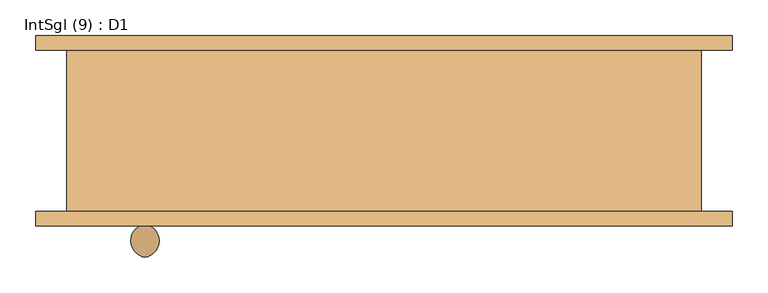
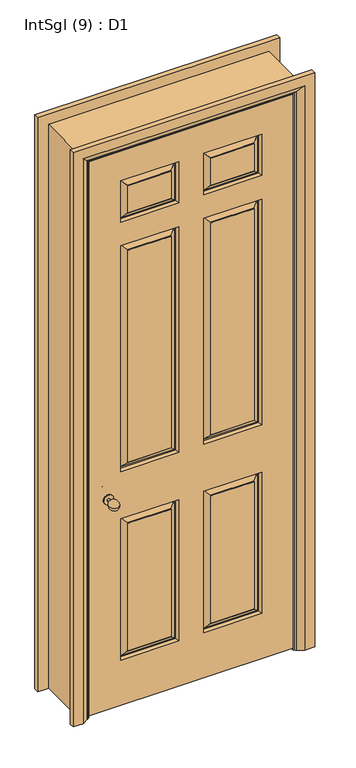
"""IFC4 building model written with IfcOpenShell, lengths in millimetres: door geometry, IntSgl (9) : D1."""

from ifc_helpers import new_model, si_unit, point, frame, origin, place, context, project, spatial, polyline, circle_curve, ellipse_curve, trimmed, outline, extrude, faceted_brep, source, transform, mapped, element, save
from ifc_brep_helpers import plane_surface, cylinder_surface, revolved_surface, advanced_brep


def intsgl_9_d1_21fcec07(model_context):
    return source(origin(), model_context, "Body", "SolidModel", [
        advanced_brep(
        [(-328.0, -55.5, 900.0), (-338.0, -55.5, 900.0), (-333.0, -11.062589, 900.0), (-328.0, -70.5, 900.0), (-338.0, -70.5, 900.0), (-353.0, -74.5, 900.0), (-313.0, -74.5, 900.0), (-353.0, -70.5, 900.0), (-313.0, -70.5, 900.0)],
        [
            (0, 1, circle_curve(frame((-333.0, -55.5, 900.0), z_axis=(0.0, 1.0, 0.0), x_axis=(-1.0, 0.0, 0.0)), 5.0)),
            (1, 2, circle_curve(frame((-329.8115138, -33.9213505, 900.0), z_axis=(0.0, 0.0, -1.0), x_axis=(0.0, -1.0, 0.0)), 23.0800654)),
            (2, 0, circle_curve(frame((-336.1884862, -33.9213505, 900.0), z_axis=(0.0, 0.0, -1.0), x_axis=(0.0, -1.0, 0.0)), 23.0800654)),
            (1, 0, circle_curve(frame((-333.0, -55.5, 900.0), z_axis=(0.0, 1.0, 0.0), x_axis=(-1.0, 0.0, 0.0)), 5.0)),
            (0, 3),
            (3, 4, circle_curve(frame((-333.0, -70.5, 900.0), z_axis=(0.0, 1.0, 0.0), x_axis=(-1.0, 0.0, 0.0)), 5.0)),
            (4, 1),
            (4, 3, circle_curve(frame((-333.0, -70.5, 900.0), z_axis=(0.0, 1.0, 0.0), x_axis=(-1.0, 0.0, 0.0)), 5.0)),
            (5, 6, circle_curve(frame((-333.0, -74.5, 900.0), z_axis=(0.0, -1.0, 0.0), x_axis=(1.0, 0.0, 0.0)), 20.0)),
            (6, 5, circle_curve(frame((-333.0, -74.5, 900.0), z_axis=(0.0, -1.0, 0.0), x_axis=(1.0, 0.0, 0.0)), 20.0)),
            (7, 8, circle_curve(frame((-333.0, -70.5, 900.0), z_axis=(0.0, 1.0, 0.0), x_axis=(1.0, 0.0, 0.0)), 20.0)),
            (8, 7, circle_curve(frame((-333.0, -70.5, 900.0), z_axis=(0.0, 1.0, 0.0), x_axis=(1.0, 0.0, 0.0)), 20.0)),
            (5, 7),
            (8, 6),
        ],
        [
            revolved_surface(trimmed(ellipse_curve(frame((-329.8115138, -33.9213505, 900.0), z_axis=(0.0, 0.0, 1.0), x_axis=(0.0, -1.0, 0.0)), 23.0800654, 23.0800654), [point((-333.0, -11.062589, 900.0))], [point((-338.0, -55.5, 900.0))], True, "CARTESIAN"), (-333.0, -70.5, 900.0), (0.0, -1.0, 0.0)),
            cylinder_surface(frame((-333.0, -70.5, 900.0), z_axis=(0.0, -1.0, 0.0), x_axis=(-1.0, 0.0, 0.0)), 5.0),
            plane_surface(frame((-313.0, -74.5, 900.0), z_axis=(0.0, -1.0, 0.0), x_axis=(0.0, 0.0, 1.0))),
            plane_surface(frame((-313.0, -70.5, 900.0), z_axis=(0.0, 1.0, 0.0), x_axis=(0.0, 0.0, -1.0))),
            cylinder_surface(frame((-333.0, -70.5, 900.0), z_axis=(0.0, -1.0, 0.0), x_axis=(1.0, 0.0, 0.0)), 20.0),
        ],
        [
            (0, [[1, 2, 3]]),
            (0, [[-2, 4, -3]]),
            (1, [[-1, 5, 6, 7]]),
            (1, [[-4, -7, 8, -5]]),
            (2, [[9, 10]]),
            (3, [[11, 12], [-6, -8]]),
            (4, [[-9, 13, -12, 14]]),
            (4, [[-10, -14, -11, -13]]),
        ],
    ),
        advanced_brep(
        [(-328.0, -131.5, 900.0), (-333.0, -175.937411, 900.0), (-338.0, -131.5, 900.0), (-338.0, -116.5, 900.0), (-328.0, -116.5, 900.0), (-353.0, -112.5, 900.0), (-313.0, -112.5, 900.0), (-353.0, -116.5, 900.0), (-313.0, -116.5, 900.0)],
        [
            (0, 1, circle_curve(frame((-336.1884862, -153.0786495, 900.0), z_axis=(0.0, 0.0, -1.0), x_axis=(0.0, 1.0, 0.0)), 23.0800654)),
            (1, 2, circle_curve(frame((-329.8115138, -153.0786495, 900.0), z_axis=(0.0, 0.0, -1.0), x_axis=(0.0, 1.0, 0.0)), 23.0800654)),
            (2, 0, circle_curve(frame((-333.0, -131.5, 900.0), z_axis=(0.0, -1.0, 0.0), x_axis=(-1.0, 0.0, 0.0)), 5.0)),
            (0, 2, circle_curve(frame((-333.0, -131.5, 900.0), z_axis=(0.0, -1.0, 0.0), x_axis=(-1.0, 0.0, 0.0)), 5.0)),
            (2, 3),
            (3, 4, circle_curve(frame((-333.0, -116.5, 900.0), z_axis=(0.0, -1.0, 0.0), x_axis=(-1.0, 0.0, 0.0)), 5.0)),
            (4, 0),
            (4, 3, circle_curve(frame((-333.0, -116.5, 900.0), z_axis=(0.0, -1.0, 0.0), x_axis=(-1.0, 0.0, 0.0)), 5.0)),
            (5, 6, circle_curve(frame((-333.0, -112.5, 900.0), z_axis=(0.0, 1.0, 0.0), x_axis=(1.0, 0.0, 0.0)), 20.0)),
            (6, 5, circle_curve(frame((-333.0, -112.5, 900.0), z_axis=(0.0, 1.0, 0.0), x_axis=(1.0, 0.0, 0.0)), 20.0)),
            (7, 8, circle_curve(frame((-333.0, -116.5, 900.0), z_axis=(0.0, -1.0, 0.0), x_axis=(1.0, 0.0, 0.0)), 20.0)),
            (8, 7, circle_curve(frame((-333.0, -116.5, 900.0), z_axis=(0.0, -1.0, 0.0), x_axis=(1.0, 0.0, 0.0)), 20.0)),
            (6, 8),
            (7, 5),
        ],
        [
            revolved_surface(trimmed(ellipse_curve(frame((-329.8115138, -153.0786495, 900.0), z_axis=(0.0, 0.0, -1.0), x_axis=(0.0, 1.0, 0.0)), 23.0800654, 23.0800654), [point((-333.0, -175.937411, 900.0))], [point((-338.0, -131.5, 900.0))], True, "CARTESIAN"), (-333.0, -116.5, 900.0), (0.0, 1.0, 0.0)),
            cylinder_surface(frame((-333.0, -116.5, 900.0), z_axis=(0.0, 1.0, 0.0), x_axis=(-1.0, 0.0, 0.0)), 5.0),
            plane_surface(frame((-313.0, -112.5, 900.0), z_axis=(0.0, 1.0, 0.0), x_axis=(0.0, 0.0, 1.0))),
            plane_surface(frame((-313.0, -116.5, 900.0), z_axis=(0.0, -1.0, 0.0), x_axis=(0.0, 0.0, -1.0))),
            cylinder_surface(frame((-333.0, -116.5, 900.0), z_axis=(0.0, 1.0, 0.0), x_axis=(1.0, 0.0, 0.0)), 20.0),
        ],
        [
            (0, [[1, 2, 3]]),
            (0, [[-1, 4, -2]]),
            (1, [[5, 6, 7, -3]]),
            (1, [[-7, 8, -5, -4]]),
            (2, [[9, 10]]),
            (3, [[11, 12], [-8, -6]]),
            (4, [[13, -11, 14, -10]]),
            (4, [[-14, -12, -13, -9]]),
        ],
    ),
        faceted_brep([(-408.0, -74.5, 2358.0), (408.0, -74.5, 2358.0), (408.0, -74.5, 8.0), (-408.0, -74.5, 8.0), (-50.0, -74.5, 800.0), (-283.0, -74.5, 800.0), (-283.0, -74.5, 200.0), (-50.0, -74.5, 200.0), (283.0, -74.5, 800.0), (50.0, -74.5, 800.0), (50.0, -74.5, 200.0), (283.0, -74.5, 200.0), (-50.0, -74.5, 1958.0), (-283.0, -74.5, 1958.0), (-283.0, -74.5, 1000.0), (-50.0, -74.5, 1000.0), (283.0, -74.5, 1958.0), (50.0, -74.5, 1958.0), (50.0, -74.5, 1000.0), (283.0, -74.5, 1000.0), (-50.0, -74.5, 2233.0), (-283.0, -74.5, 2233.0), (-283.0, -74.5, 2058.0), (-50.0, -74.5, 2058.0), (283.0, -74.5, 2233.0), (50.0, -74.5, 2233.0), (50.0, -74.5, 2058.0), (283.0, -74.5, 2058.0), (-80.0, -74.5, 230.0), (-253.0, -74.5, 230.0), (-253.0, -74.5, 770.0), (-80.0, -74.5, 770.0), (253.0, -74.5, 230.0), (80.0, -74.5, 230.0), (80.0, -74.5, 770.0), (253.0, -74.5, 770.0), (-80.0, -74.5, 1030.0), (-253.0, -74.5, 1030.0), (-253.0, -74.5, 1928.0), (-80.0, -74.5, 1928.0), (253.0, -74.5, 1030.0), (80.0, -74.5, 1030.0), (80.0, -74.5, 1928.0), (253.0, -74.5, 1928.0), (-80.0, -74.5, 2088.0), (-253.0, -74.5, 2088.0), (-253.0, -74.5, 2203.0), (-80.0, -74.5, 2203.0), (253.0, -74.5, 2088.0), (80.0, -74.5, 2088.0), (80.0, -74.5, 2203.0), (253.0, -74.5, 2203.0), (-408.0, -112.5, 2358.0), (-408.0, -112.5, 8.0), (408.0, -112.5, 8.0), (408.0, -112.5, 2358.0), (50.0, -112.5, 800.0), (283.0, -112.5, 800.0), (283.0, -112.5, 200.0), (50.0, -112.5, 200.0), (-283.0, -112.5, 800.0), (-50.0, -112.5, 800.0), (-50.0, -112.5, 200.0), (-283.0, -112.5, 200.0), (50.0, -112.5, 1958.0), (283.0, -112.5, 1958.0), (283.0, -112.5, 1000.0), (50.0, -112.5, 1000.0), (-283.0, -112.5, 1958.0), (-50.0, -112.5, 1958.0), (-50.0, -112.5, 1000.0), (-283.0, -112.5, 1000.0), (50.0, -112.5, 2233.0), (283.0, -112.5, 2233.0), (283.0, -112.5, 2058.0), (50.0, -112.5, 2058.0), (-283.0, -112.5, 2233.0), (-50.0, -112.5, 2233.0), (-50.0, -112.5, 2058.0), (-283.0, -112.5, 2058.0), (80.0, -112.5, 230.0), (253.0, -112.5, 230.0), (253.0, -112.5, 770.0), (80.0, -112.5, 770.0), (-253.0, -112.5, 230.0), (-80.0, -112.5, 230.0), (-80.0, -112.5, 770.0), (-253.0, -112.5, 770.0), (80.0, -112.5, 1030.0), (253.0, -112.5, 1030.0), (253.0, -112.5, 1928.0), (80.0, -112.5, 1928.0), (-253.0, -112.5, 1030.0), (-80.0, -112.5, 1030.0), (-80.0, -112.5, 1928.0), (-253.0, -112.5, 1928.0), (80.0, -112.5, 2088.0), (253.0, -112.5, 2088.0), (253.0, -112.5, 2203.0), (80.0, -112.5, 2203.0), (-253.0, -112.5, 2088.0), (-80.0, -112.5, 2088.0), (-80.0, -112.5, 2203.0), (-253.0, -112.5, 2203.0), (80.0, -111.5, 230.0), (80.0, -111.5, 770.0), (58.0, -97.5, 208.0), (78.0, -111.5, 228.0), (78.0, -111.5, 772.0), (58.0, -97.5, 792.0), (53.0, -97.5, 203.0), (53.0, -97.5, 797.0), (253.0, -111.5, 770.0), (255.0, -111.5, 772.0), (275.0, -97.5, 792.0), (280.0, -97.5, 797.0), (253.0, -111.5, 230.0), (255.0, -111.5, 228.0), (275.0, -97.5, 208.0), (280.0, -97.5, 203.0), (-253.0, -111.5, 230.0), (-253.0, -111.5, 770.0), (-275.0, -97.5, 208.0), (-255.0, -111.5, 228.0), (-255.0, -111.5, 772.0), (-275.0, -97.5, 792.0), (-280.0, -97.5, 203.0), (-280.0, -97.5, 797.0), (-80.0, -111.5, 770.0), (-78.0, -111.5, 772.0), (-58.0, -97.5, 792.0), (-53.0, -97.5, 797.0), (-80.0, -111.5, 230.0), (-78.0, -111.5, 228.0), (-58.0, -97.5, 208.0), (-53.0, -97.5, 203.0), (80.0, -111.5, 1030.0), (80.0, -111.5, 1928.0), (58.0, -97.5, 1008.0), (78.0, -111.5, 1028.0), (78.0, -111.5, 1930.0), (58.0, -97.5, 1950.0), (53.0, -97.5, 1003.0), (53.0, -97.5, 1955.0), (253.0, -111.5, 1928.0), (255.0, -111.5, 1930.0), (275.0, -97.5, 1950.0), (280.0, -97.5, 1955.0), (253.0, -111.5, 1030.0), (255.0, -111.5, 1028.0), (275.0, -97.5, 1008.0), (280.0, -97.5, 1003.0), (-253.0, -111.5, 1030.0), (-253.0, -111.5, 1928.0), (-275.0, -97.5, 1008.0), (-255.0, -111.5, 1028.0), (-255.0, -111.5, 1930.0), (-275.0, -97.5, 1950.0), (-280.0, -97.5, 1003.0), (-280.0, -97.5, 1955.0), (-80.0, -111.5, 1928.0), (-78.0, -111.5, 1930.0), (-58.0, -97.5, 1950.0), (-53.0, -97.5, 1955.0), (-80.0, -111.5, 1030.0), (-78.0, -111.5, 1028.0), (-58.0, -97.5, 1008.0), (-53.0, -97.5, 1003.0), (80.0, -111.5, 2088.0), (80.0, -111.5, 2203.0), (58.0, -97.5, 2066.0), (78.0, -111.5, 2086.0), (78.0, -111.5, 2205.0), (58.0, -97.5, 2225.0), (53.0, -97.5, 2061.0), (53.0, -97.5, 2230.0), (253.0, -111.5, 2203.0), (255.0, -111.5, 2205.0), (275.0, -97.5, 2225.0), (280.0, -97.5, 2230.0), (253.0, -111.5, 2088.0), (255.0, -111.5, 2086.0), (275.0, -97.5, 2066.0), (280.0, -97.5, 2061.0), (-253.0, -111.5, 2088.0), (-253.0, -111.5, 2203.0), (-275.0, -97.5, 2066.0), (-255.0, -111.5, 2086.0), (-255.0, -111.5, 2205.0), (-275.0, -97.5, 2225.0), (-280.0, -97.5, 2061.0), (-280.0, -97.5, 2230.0), (-80.0, -111.5, 2203.0), (-78.0, -111.5, 2205.0), (-58.0, -97.5, 2225.0), (-53.0, -97.5, 2230.0), (-80.0, -111.5, 2088.0), (-78.0, -111.5, 2086.0), (-58.0, -97.5, 2066.0), (-53.0, -97.5, 2061.0), (-80.0, -75.5, 230.0), (-80.0, -75.5, 770.0), (-58.0, -89.5, 208.0), (-78.0, -75.5, 228.0), (-78.0, -75.5, 772.0), (-58.0, -89.5, 792.0), (-53.0, -89.5, 203.0), (-53.0, -89.5, 797.0), (-253.0, -75.5, 770.0), (-255.0, -75.5, 772.0), (-275.0, -89.5, 792.0), (-280.0, -89.5, 797.0), (-253.0, -75.5, 230.0), (-255.0, -75.5, 228.0), (-275.0, -89.5, 208.0), (-280.0, -89.5, 203.0), (253.0, -75.5, 230.0), (253.0, -75.5, 770.0), (275.0, -89.5, 208.0), (255.0, -75.5, 228.0), (255.0, -75.5, 772.0), (275.0, -89.5, 792.0), (280.0, -89.5, 203.0), (280.0, -89.5, 797.0), (80.0, -75.5, 770.0), (78.0, -75.5, 772.0), (58.0, -89.5, 792.0), (53.0, -89.5, 797.0), (80.0, -75.5, 230.0), (78.0, -75.5, 228.0), (58.0, -89.5, 208.0), (53.0, -89.5, 203.0), (-80.0, -75.5, 1030.0), (-80.0, -75.5, 1928.0), (-58.0, -89.5, 1008.0), (-78.0, -75.5, 1028.0), (-78.0, -75.5, 1930.0), (-58.0, -89.5, 1950.0), (-53.0, -89.5, 1003.0), (-53.0, -89.5, 1955.0), (-253.0, -75.5, 1928.0), (-255.0, -75.5, 1930.0), (-275.0, -89.5, 1950.0), (-280.0, -89.5, 1955.0), (-253.0, -75.5, 1030.0), (-255.0, -75.5, 1028.0), (-275.0, -89.5, 1008.0), (-280.0, -89.5, 1003.0), (253.0, -75.5, 1030.0), (253.0, -75.5, 1928.0), (275.0, -89.5, 1008.0), (255.0, -75.5, 1028.0), (255.0, -75.5, 1930.0), (275.0, -89.5, 1950.0), (280.0, -89.5, 1003.0), (280.0, -89.5, 1955.0), (80.0, -75.5, 1928.0), (78.0, -75.5, 1930.0), (58.0, -89.5, 1950.0), (53.0, -89.5, 1955.0), (80.0, -75.5, 1030.0), (78.0, -75.5, 1028.0), (58.0, -89.5, 1008.0), (53.0, -89.5, 1003.0), (-80.0, -75.5, 2088.0), (-80.0, -75.5, 2203.0), (-58.0, -89.5, 2066.0), (-78.0, -75.5, 2086.0), (-78.0, -75.5, 2205.0), (-58.0, -89.5, 2225.0), (-53.0, -89.5, 2061.0), (-53.0, -89.5, 2230.0), (-253.0, -75.5, 2203.0), (-255.0, -75.5, 2205.0), (-275.0, -89.5, 2225.0), (-280.0, -89.5, 2230.0), (-253.0, -75.5, 2088.0), (-255.0, -75.5, 2086.0), (-275.0, -89.5, 2066.0), (-280.0, -89.5, 2061.0), (253.0, -75.5, 2088.0), (253.0, -75.5, 2203.0), (275.0, -89.5, 2066.0), (255.0, -75.5, 2086.0), (255.0, -75.5, 2205.0), (275.0, -89.5, 2225.0), (280.0, -89.5, 2061.0), (280.0, -89.5, 2230.0), (80.0, -75.5, 2203.0), (78.0, -75.5, 2205.0), (58.0, -89.5, 2225.0), (53.0, -89.5, 2230.0), (80.0, -75.5, 2088.0), (78.0, -75.5, 2086.0), (58.0, -89.5, 2066.0), (53.0, -89.5, 2061.0)], [[[0, 1, 2, 3], [4, 5, 6, 7], [8, 9, 10, 11], [12, 13, 14, 15], [16, 17, 18, 19], [20, 21, 22, 23], [24, 25, 26, 27]], [[28, 29, 30, 31]], [[32, 33, 34, 35]], [[36, 37, 38, 39]], [[40, 41, 42, 43]], [[44, 45, 46, 47]], [[48, 49, 50, 51]], [[52, 53, 54, 55], [56, 57, 58, 59], [60, 61, 62, 63], [64, 65, 66, 67], [68, 69, 70, 71], [72, 73, 74, 75], [76, 77, 78, 79]], [[80, 81, 82, 83]], [[84, 85, 86, 87]], [[88, 89, 90, 91]], [[92, 93, 94, 95]], [[96, 97, 98, 99]], [[100, 101, 102, 103]], [[3, 53, 52, 0]], [[2, 54, 53, 3]], [[1, 55, 54, 2]], [[0, 52, 55, 1]], [[104, 80, 83, 105]], [[106, 107, 108, 109]], [[56, 59, 110, 111]], [[83, 82, 112, 105]], [[108, 113, 114, 109]], [[111, 115, 57, 56]], [[82, 81, 116, 112]], [[113, 117, 118, 114]], [[115, 119, 58, 57]], [[104, 116, 81, 80]], [[107, 117, 113, 108], [105, 112, 116, 104]], [[106, 118, 117, 107]], [[110, 119, 115, 111], [109, 114, 118, 106]], [[59, 58, 119, 110]], [[120, 84, 87, 121]], [[122, 123, 124, 125]], [[60, 63, 126, 127]], [[87, 86, 128, 121]], [[124, 129, 130, 125]], [[127, 131, 61, 60]], [[86, 85, 132, 128]], [[129, 133, 134, 130]], [[131, 135, 62, 61]], [[120, 132, 85, 84]], [[123, 133, 129, 124], [121, 128, 132, 120]], [[122, 134, 133, 123]], [[126, 135, 131, 127], [125, 130, 134, 122]], [[63, 62, 135, 126]], [[136, 88, 91, 137]], [[138, 139, 140, 141]], [[64, 67, 142, 143]], [[91, 90, 144, 137]], [[140, 145, 146, 141]], [[143, 147, 65, 64]], [[90, 89, 148, 144]], [[145, 149, 150, 146]], [[147, 151, 66, 65]], [[136, 148, 89, 88]], [[139, 149, 145, 140], [137, 144, 148, 136]], [[138, 150, 149, 139]], [[142, 151, 147, 143], [141, 146, 150, 138]], [[67, 66, 151, 142]], [[152, 92, 95, 153]], [[154, 155, 156, 157]], [[68, 71, 158, 159]], [[95, 94, 160, 153]], [[156, 161, 162, 157]], [[159, 163, 69, 68]], [[94, 93, 164, 160]], [[161, 165, 166, 162]], [[163, 167, 70, 69]], [[152, 164, 93, 92]], [[155, 165, 161, 156], [153, 160, 164, 152]], [[154, 166, 165, 155]], [[158, 167, 163, 159], [157, 162, 166, 154]], [[71, 70, 167, 158]], [[168, 96, 99, 169]], [[170, 171, 172, 173]], [[72, 75, 174, 175]], [[99, 98, 176, 169]], [[172, 177, 178, 173]], [[175, 179, 73, 72]], [[98, 97, 180, 176]], [[177, 181, 182, 178]], [[179, 183, 74, 73]], [[168, 180, 97, 96]], [[171, 181, 177, 172], [169, 176, 180, 168]], [[170, 182, 181, 171]], [[174, 183, 179, 175], [173, 178, 182, 170]], [[75, 74, 183, 174]], [[184, 100, 103, 185]], [[186, 187, 188, 189]], [[76, 79, 190, 191]], [[103, 102, 192, 185]], [[188, 193, 194, 189]], [[191, 195, 77, 76]], [[102, 101, 196, 192]], [[193, 197, 198, 194]], [[195, 199, 78, 77]], [[184, 196, 101, 100]], [[187, 197, 193, 188], [185, 192, 196, 184]], [[186, 198, 197, 187]], [[190, 199, 195, 191], [189, 194, 198, 186]], [[79, 78, 199, 190]], [[200, 28, 31, 201]], [[202, 203, 204, 205]], [[4, 7, 206, 207]], [[31, 30, 208, 201]], [[204, 209, 210, 205]], [[207, 211, 5, 4]], [[30, 29, 212, 208]], [[209, 213, 214, 210]], [[211, 215, 6, 5]], [[200, 212, 29, 28]], [[203, 213, 209, 204], [201, 208, 212, 200]], [[202, 214, 213, 203]], [[206, 215, 211, 207], [205, 210, 214, 202]], [[7, 6, 215, 206]], [[216, 32, 35, 217]], [[218, 219, 220, 221]], [[8, 11, 222, 223]], [[35, 34, 224, 217]], [[220, 225, 226, 221]], [[223, 227, 9, 8]], [[34, 33, 228, 224]], [[225, 229, 230, 226]], [[227, 231, 10, 9]], [[216, 228, 33, 32]], [[219, 229, 225, 220], [217, 224, 228, 216]], [[218, 230, 229, 219]], [[222, 231, 227, 223], [221, 226, 230, 218]], [[11, 10, 231, 222]], [[232, 36, 39, 233]], [[234, 235, 236, 237]], [[12, 15, 238, 239]], [[39, 38, 240, 233]], [[236, 241, 242, 237]], [[239, 243, 13, 12]], [[38, 37, 244, 240]], [[241, 245, 246, 242]], [[243, 247, 14, 13]], [[232, 244, 37, 36]], [[235, 245, 241, 236], [233, 240, 244, 232]], [[234, 246, 245, 235]], [[238, 247, 243, 239], [237, 242, 246, 234]], [[15, 14, 247, 238]], [[248, 40, 43, 249]], [[250, 251, 252, 253]], [[16, 19, 254, 255]], [[43, 42, 256, 249]], [[252, 257, 258, 253]], [[255, 259, 17, 16]], [[42, 41, 260, 256]], [[257, 261, 262, 258]], [[259, 263, 18, 17]], [[248, 260, 41, 40]], [[251, 261, 257, 252], [249, 256, 260, 248]], [[250, 262, 261, 251]], [[254, 263, 259, 255], [253, 258, 262, 250]], [[19, 18, 263, 254]], [[264, 44, 47, 265]], [[266, 267, 268, 269]], [[20, 23, 270, 271]], [[47, 46, 272, 265]], [[268, 273, 274, 269]], [[271, 275, 21, 20]], [[46, 45, 276, 272]], [[273, 277, 278, 274]], [[275, 279, 22, 21]], [[264, 276, 45, 44]], [[267, 277, 273, 268], [265, 272, 276, 264]], [[266, 278, 277, 267]], [[270, 279, 275, 271], [269, 274, 278, 266]], [[23, 22, 279, 270]], [[280, 48, 51, 281]], [[282, 283, 284, 285]], [[24, 27, 286, 287]], [[51, 50, 288, 281]], [[284, 289, 290, 285]], [[287, 291, 25, 24]], [[50, 49, 292, 288]], [[289, 293, 294, 290]], [[291, 295, 26, 25]], [[280, 292, 49, 48]], [[283, 293, 289, 284], [281, 288, 292, 280]], [[282, 294, 293, 283]], [[286, 295, 291, 287], [285, 290, 294, 282]], [[27, 26, 295, 286]]]),
        faceted_brep([(-410.0, -112.5, 0.0), (-442.0, -112.5, 0.0), (-442.0, 112.5, 0.0), (-410.0, 112.5, 0.0), (-410.0, 112.5, 2360.0), (-410.0, -112.5, 2360.0), (-442.0, 112.5, 2392.0), (-442.0, -112.5, 2392.0), (410.0, -112.5, 0.0), (410.0, 112.5, 0.0), (442.0, 112.5, 0.0), (442.0, -112.5, 0.0), (410.0, -112.5, 2360.0), (442.0, -112.5, 2392.0), (442.0, 112.5, 2392.0), (410.0, 112.5, 2360.0)], [[[0, 1, 2, 3]], [[3, 4, 5, 0]], [[2, 6, 4, 3]], [[1, 7, 6, 2]], [[0, 5, 7, 1]], [[8, 9, 10, 11]], [[12, 8, 11, 13]], [[13, 11, 10, 14]], [[14, 10, 9, 15]], [[15, 9, 8, 12]], [[4, 15, 12, 5]], [[6, 14, 15, 4]], [[7, 13, 14, 6]], [[5, 12, 13, 7]]]),
        extrude(outline(polyline([(0.0, -391.0), (2341.0, -391.0), (2341.0, 391.0), (0.0, 391.0), (0.0, 410.0), (2360.0, 410.0), (2360.0, -410.0), (0.0, -410.0), (0.0, -391.0)])), frame((0.0, -72.5, 0.0), z_axis=(0.0, 1.0, 0.0), x_axis=(0.0, 0.0, 1.0)), (0.0, 0.0, 1.0), 32.0),
        advanced_brep(
        [(-485.0, 132.5, 0.0), (-445.0, 132.5, 0.0), (-419.0, 118.5, 0.0), (-415.0, 112.5, 0.0), (-485.0, 112.5, 0.0), (-485.0, 112.5, 2435.0), (-485.0, 132.5, 2435.0), (-415.0, 112.5, 2365.0), (415.0, 112.5, 2365.0), (415.0, 112.5, 0.0), (485.0, 112.5, 0.0), (485.0, 112.5, 2435.0), (-419.0, 118.5, 2369.0), (-445.0, 132.5, 2395.0), (485.0, 132.5, 2435.0), (485.0, 132.5, 0.0), (445.0, 132.5, 0.0), (445.0, 132.5, 2395.0), (419.0, 118.5, 0.0), (419.0, 118.5, 2369.0)],
        [
            (0, 1),
            (1, 2),
            (2, 3, circle_curve(frame((-423.0, 111.5, 0.0), z_axis=(0.0, 0.0, -1.0), x_axis=(-1.0, 0.0, 0.0)), 8.0622577)),
            (3, 4),
            (4, 0),
            (4, 5),
            (5, 6),
            (6, 0),
            (3, 7),
            (7, 8),
            (8, 9),
            (9, 10),
            (10, 11),
            (11, 5),
            (2, 12),
            (12, 7, ellipse_curve(frame((-423.0, 111.5, 2373.0), z_axis=(-0.7071067811865475, 0.0, -0.7071067811865475), x_axis=(0.7071067811865474, 0.0, -0.7071067811865476)), 11.4017543, 8.0622577)),
            (1, 13),
            (13, 12),
            (6, 14),
            (14, 15),
            (15, 16),
            (16, 17),
            (17, 13),
            (10, 15),
            (14, 11),
            (9, 18, circle_curve(frame((423.0, 111.5, 0.0), z_axis=(0.0, 0.0, -1.0), x_axis=(1.0, 0.0, 0.0)), 8.0622577)),
            (18, 16),
            (19, 18),
            (8, 19, ellipse_curve(frame((423.0, 111.5, 2373.0), z_axis=(0.7071067811865475, 0.0, -0.7071067811865475), x_axis=(0.7071067811865474, 0.0, 0.7071067811865476)), 11.4017543, 8.0622577)),
            (19, 17),
            (12, 19),
        ],
        [
            plane_surface(frame((-415.0, 112.5, 0.0), z_axis=(0.0, 0.0, -1.0), x_axis=(0.0, 1.0, 0.0))),
            plane_surface(frame((-485.0, 132.5, 0.0), z_axis=(-1.0, 0.0, 0.0), x_axis=(0.0, 0.0, 1.0))),
            plane_surface(frame((-485.0, 112.5, 0.0), z_axis=(0.0, -1.0, 0.0), x_axis=(0.0, 0.0, 1.0))),
            cylinder_surface(frame((-423.0, 111.5, 0.0), z_axis=(0.0, 0.0, -1.0), x_axis=(-1.0, 0.0, 0.0)), 8.0622577),
            plane_surface(frame((-419.0, 118.5, 0.0), z_axis=(0.4740998230350183, 0.8804710999221749, 0.0), x_axis=(0.0, 0.0, 1.0))),
            plane_surface(frame((-445.0, 132.5, 0.0), z_axis=(0.0, 1.0, 0.0), x_axis=(0.0, 0.0, 1.0))),
            plane_surface(frame((485.0, 132.5, 2435.0), z_axis=(1.0, 0.0, 0.0), x_axis=(0.0, 0.0, -1.0))),
            plane_surface(frame((415.0, 112.5, 0.0), z_axis=(0.0, 0.0, -1.0), x_axis=(0.0, 1.0, 0.0))),
            cylinder_surface(frame((423.0, 111.5, 2365.0), z_axis=(0.0, 0.0, 1.0), x_axis=(1.0, 0.0, 0.0)), 8.0622577),
            plane_surface(frame((419.0, 118.5, 2369.0), z_axis=(-0.4740998230350183, 0.8804710999221749, 0.0), x_axis=(0.0, 0.0, -1.0))),
            plane_surface(frame((-485.0, 132.5, 2435.0), z_axis=(0.0, 0.0, 1.0), x_axis=(1.0, 0.0, 0.0))),
            cylinder_surface(frame((-415.0, 111.5, 2373.0), z_axis=(-1.0, 0.0, 0.0), x_axis=(0.0, 0.0, 1.0)), 8.0622577),
            plane_surface(frame((-419.0, 118.5, 2369.0), z_axis=(0.0, 0.8804710999221749, -0.4740998230350183), x_axis=(1.0, 0.0, 0.0))),
        ],
        [
            (0, [[1, 2, 3, 4, 5]]),
            (1, [[6, 7, 8, -5]]),
            (2, [[9, 10, 11, 12, 13, 14, -6, -4]]),
            (3, [[15, 16, -9, -3]]),
            (4, [[17, 18, -15, -2]]),
            (5, [[-8, 19, 20, 21, 22, 23, -17, -1]]),
            (6, [[-13, 24, -20, 25]]),
            (7, [[-24, -12, 26, 27, -21]]),
            (8, [[28, -26, -11, 29]]),
            (9, [[-22, -27, -28, 30]]),
            (10, [[-14, -25, -19, -7]]),
            (11, [[31, -29, -10, -16]]),
            (12, [[-23, -30, -31, -18]]),
        ],
    ),
        advanced_brep(
        [(485.0, -132.5, 0.0), (445.0, -132.5, 0.0), (419.0, -118.5, 0.0), (415.0, -112.5, 0.0), (485.0, -112.5, 0.0), (485.0, -112.5, 2435.0), (485.0, -132.5, 2435.0), (415.0, -112.5, 2365.0), (-415.0, -112.5, 2365.0), (-415.0, -112.5, 0.0), (-485.0, -112.5, 0.0), (-485.0, -112.5, 2435.0), (419.0, -118.5, 2369.0), (445.0, -132.5, 2395.0), (-485.0, -132.5, 2435.0), (-485.0, -132.5, 0.0), (-445.0, -132.5, 0.0), (-445.0, -132.5, 2395.0), (-419.0, -118.5, 0.0), (-419.0, -118.5, 2369.0)],
        [
            (0, 1),
            (1, 2),
            (2, 3, circle_curve(frame((423.0, -111.5, 0.0), z_axis=(0.0, 0.0, -1.0), x_axis=(1.0, 0.0, 0.0)), 8.0622577)),
            (3, 4),
            (4, 0),
            (4, 5),
            (5, 6),
            (6, 0),
            (3, 7),
            (7, 8),
            (8, 9),
            (9, 10),
            (10, 11),
            (11, 5),
            (2, 12),
            (12, 7, ellipse_curve(frame((423.0, -111.5, 2373.0), z_axis=(0.7071067811865475, 0.0, -0.7071067811865475), x_axis=(-0.7071067811865474, 0.0, -0.7071067811865476)), 11.4017543, 8.0622577)),
            (1, 13),
            (13, 12),
            (6, 14),
            (14, 15),
            (15, 16),
            (16, 17),
            (17, 13),
            (10, 15),
            (14, 11),
            (9, 18, circle_curve(frame((-423.0, -111.5, 0.0), z_axis=(0.0, 0.0, -1.0), x_axis=(-1.0, 0.0, 0.0)), 8.0622577)),
            (18, 16),
            (19, 18),
            (8, 19, ellipse_curve(frame((-423.0, -111.5, 2373.0), z_axis=(-0.7071067811865475, 0.0, -0.7071067811865475), x_axis=(-0.7071067811865474, 0.0, 0.7071067811865476)), 11.4017543, 8.0622577)),
            (19, 17),
            (12, 19),
        ],
        [
            plane_surface(frame((415.0, -112.5, 0.0), z_axis=(0.0, 0.0, -1.0), x_axis=(0.0, -1.0, 0.0))),
            plane_surface(frame((485.0, -132.5, 0.0), z_axis=(1.0, 0.0, 0.0), x_axis=(0.0, 0.0, 1.0))),
            plane_surface(frame((485.0, -112.5, 0.0), z_axis=(0.0, 1.0, 0.0), x_axis=(0.0, 0.0, 1.0))),
            cylinder_surface(frame((423.0, -111.5, 0.0), z_axis=(0.0, 0.0, -1.0), x_axis=(1.0, 0.0, 0.0)), 8.0622577),
            plane_surface(frame((419.0, -118.5, 0.0), z_axis=(-0.4740998230350183, -0.8804710999221749, 0.0), x_axis=(0.0, 0.0, 1.0))),
            plane_surface(frame((445.0, -132.5, 0.0), z_axis=(0.0, -1.0, 0.0), x_axis=(0.0, 0.0, 1.0))),
            plane_surface(frame((-485.0, -132.5, 2435.0), z_axis=(-1.0, 0.0, 0.0), x_axis=(0.0, 0.0, -1.0))),
            plane_surface(frame((-415.0, -112.5, 0.0), z_axis=(0.0, 0.0, -1.0), x_axis=(0.0, -1.0, 0.0))),
            cylinder_surface(frame((-423.0, -111.5, 2365.0), z_axis=(0.0, 0.0, 1.0), x_axis=(-1.0, 0.0, 0.0)), 8.0622577),
            plane_surface(frame((-419.0, -118.5, 2369.0), z_axis=(0.4740998230350183, -0.8804710999221749, 0.0), x_axis=(0.0, 0.0, -1.0))),
            plane_surface(frame((485.0, -132.5, 2435.0), z_axis=(0.0, 0.0, 1.0), x_axis=(-1.0, 0.0, 0.0))),
            cylinder_surface(frame((415.0, -111.5, 2373.0), z_axis=(1.0, 0.0, 0.0), x_axis=(0.0, 0.0, 1.0)), 8.0622577),
            plane_surface(frame((419.0, -118.5, 2369.0), z_axis=(0.0, -0.8804710999221749, -0.4740998230350183), x_axis=(-1.0, 0.0, 0.0))),
        ],
        [
            (0, [[1, 2, 3, 4, 5]]),
            (1, [[6, 7, 8, -5]]),
            (2, [[9, 10, 11, 12, 13, 14, -6, -4]]),
            (3, [[15, 16, -9, -3]]),
            (4, [[17, 18, -15, -2]]),
            (5, [[-8, 19, 20, 21, 22, 23, -17, -1]]),
            (6, [[-13, 24, -20, 25]]),
            (7, [[-24, -12, 26, 27, -21]]),
            (8, [[28, -26, -11, 29]]),
            (9, [[-22, -27, -28, 30]]),
            (10, [[-14, -25, -19, -7]]),
            (11, [[31, -29, -10, -16]]),
            (12, [[-23, -30, -31, -18]]),
        ],
    ),
    ])


if __name__ == "__main__":
    model = new_model("IFC4")
    model_context = context("Model", 3, world=origin())
    ifc_project = project(units=[si_unit("LENGTHUNIT", "METRE", prefix="MILLI")], contexts=[model_context])
    site = spatial("IfcSite", under=ifc_project)
    building = spatial("IfcBuilding", under=site)
    placement = place(None, origin())
    intsgl_9_d1_shape = intsgl_9_d1_21fcec07(model_context)
    element("IfcDoor", 1, ObjectType="IntSgl (9) : D1", at=placement, inside=building, context=model_context, shape_type="MappedRepresentation", body=[
        mapped(intsgl_9_d1_shape, transform((0.0, 0.0, 0.0), x_axis=(1.0, 0.0, 0.0), y_axis=(0.0, 1.0, 0.0), z_axis=(0.0, 0.0, 1.0))),
    ])
    save(model, "model.ifc")

# Revit data of these elements
# Type "IntSgl (9) : D1"
#   Type Mark = "49"
#   Operation = "SingleSwingRight"
#   Manufacturer = "Revit"
#   Keynote = "L20"
#   UnderCut = 8 mm
#   Tolerance = 2 mm
#   Thickness = 38 mm
#   Structural Tolerance = 8 mm
#   StopDepth = 32 mm
#   Stop Thickness = 19 mm
#   Stile Top Rail = 125 mm
#   Stile Shutting = 125 mm
#   Stile Muntin Rail = 100 mm
#   Stile Lock Rail = 200 mm
#   Stile Intermediate/Frieze = 100 mm
#   Stile Hanging = 125 mm
#   Stile Bottom Rail = 200 mm
#   Rough Width = 900 mm
#   Rough Height = 2400 mm
#   Height to Top Lock Rail = 1000 mm
#   Handle Z Distance = 900 mm
#   Handle X Distance = 75 mm
#   Frame Thickness = 32 mm
#   Door Panel Width = 816 mm
#   Height = 2400 mm
#   Width = 900 mm
#   Door Panel Thickness = 38 mm
#   Door Panel Offset = 0 mm
#   Door Panel Height = 2350 mm
#   Architrave Setback = 5 mm
#   Vis - Ironmongery = yes
#   Material Ironmongery = Door - Handle
#   Material Frame = Door - Frame/Mullion
#   Material Door = Door - Panel
#   Material Architrave = Door - Architrave
#   Function = (empty or 0)
#   Wall Closure = (empty or 0)
# Element 1 (IfcDoor, "IntSgl (9) : D1")
#   Materials on its faces: "Door - Panel", "Door - Architrave", "Door - Frame/Mullion", "Door - Handle"
# Materials
#   "Door - Handle": colour RGB 0 0 0, transparency 0, Keynote = "P21", Cost = 0, Export to IFC = 0
#   "Door - Frame/Mullion": class "Wood", colour RGB 212 179 113, transparency 0, Keynote = "L20", Cost = 0, Export to IFC = 0
#   "Door - Panel": class "Wood", colour RGB 210 159 95, transparency 0, Keynote = "L20", Cost = 0, Export to IFC = 0
#   "Door - Architrave": class "Wood", colour RGB 154 90 5, transparency 0, Keynote = "P20", Cost = 0, Export to IFC = 0
